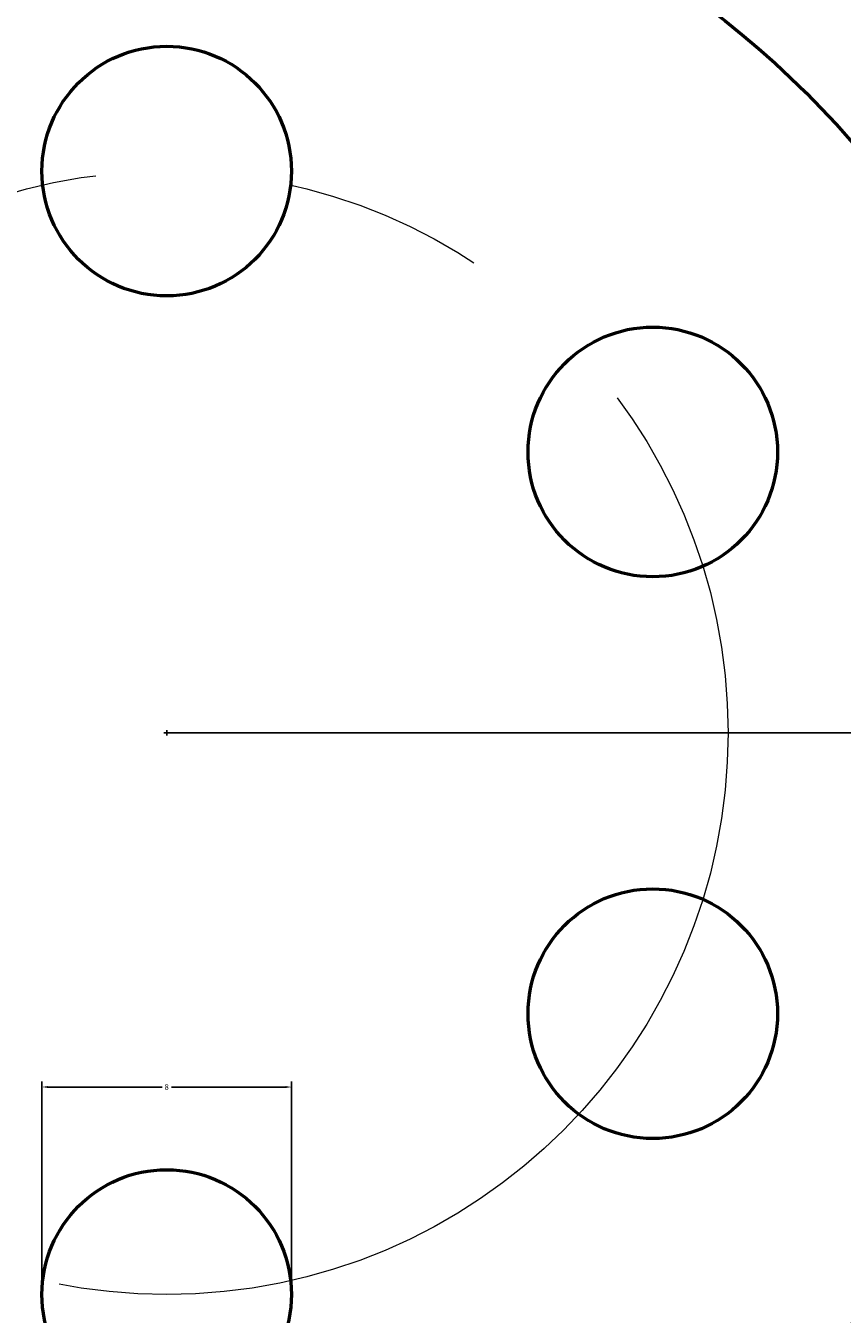
# Model space of a CAD drawing. Units: inches. Extents: x -11 to 126, y -62 to 82.
# Tile 4 of 10: x 55 to 81, y -40 to 1. Entities that reach past the tile are written whole.
import ezdxf

# ---------------------------------------------------------------- set-up
doc = ezdxf.new("R2010")
doc.units = ezdxf.units.IN
doc.header["$MEASUREMENT"] = 0
doc.linetypes.add('CENTER', pattern=[50.8, 31.75, -6.35, 6.35, -6.35])
for name, color, linetype, lineweight in [('M-CNTR', 4, 'CENTER', 18), ('M-DIMS', 2, 'Continuous', 18), ('M-OUTL', 7, 'Continuous', 50)]:
    doc.layers.add(name, color=color, linetype=linetype, lineweight=lineweight)
doc.styles.get("Standard").update_dxf_attribs({"font": 'arial.ttf'})
doc.dimstyles.get("Standard").update_dxf_attribs({"dimtxt": 0.18, "dimasz": 0.18, "dimexe": 0.18, "dimexo": 0.0625, "dimgap": 0.09, "dimtad": 0, "dimtih": 1, "dimtoh": 1, "dimdec": 4, "dimzin": 0, "dimdsep": 46, "dimtxsty": 'Standard', "dimcen": 0.09, "dimadec": 0, "dimazin": 0, "dimtfac": 1, "dimtdec": 4, "dimtofl": 0, "dimtmove": 0, "dimatfit": 3, "dimfxl": 1, "dimtolj": 1, "dimtzin": 0, "dimarcsym": 0})

# ---------------------------------------------------------------- blocks, each defined once
blk = doc.blocks.new('*U3')
blk.add_circle((0, 0), 4)
blk = doc.blocks.new('*U4')
at = {"layer": 'M-OUTL', "color": 0, "linetype": 'ByBlock', "lineweight": -2, "transparency": 16777216}
blk.add_blockref('*U3', (59.232, -3.646), dxfattribs=at)
for p, rotation in [((74.82, -12.646), 300), ((74.82, -30.646), 240), ((59.232, -39.646), 180)]:
    blk.add_blockref('*U3', p, dxfattribs=dict(at, rotation=rotation))
blk = doc.blocks.new('*D5')
at = {"layer": 'Defpoints', "color": 0, "transparency": 16777216}
for p in [(119.232, 12.354), (-0.749, 11.479), (119.232, -57.296)]:
    blk.add_point(p, dxfattribs=at)
at = {"layer": 'M-DIMS', "color": 0, "lineweight": -2, "transparency": 16777216}
for p, q in [((119.232, 12.292), (119.232, -57.476)), ((-0.749, 11.416), (-0.749, -57.476)), ((-0.569, -57.296), (58.786, -57.296)), ((119.052, -57.296), (59.696, -57.296))]:
    blk.add_line(p, q, dxfattribs=at)
at = {"layer": 'M-DIMS', "color": 0, "transparency": 16777216}
for points in [[(-0.569, -57.266), (-0.569, -57.326), (-0.749, -57.296)], [(119.052, -57.266), (119.052, -57.326), (119.232, -57.296)]]:
    blk.add_solid(points, dxfattribs=at)
at = {"layer": 'M-DIMS', "color": 0, "transparency": 16777216, "insert": (59.241, -57.296), "char_height": 0.18, "attachment_point": 5}
blk.add_mtext('\\A1;119.98', dxfattribs=at)
blk = doc.blocks.new('*D6')
at = {"layer": 'Defpoints', "color": 0, "transparency": 16777216}
for p in [(-7.399, 75.354), (59.232, 75.354), (59.232, -50.646)]:
    blk.add_point(p, dxfattribs=at)
at = {"layer": 'M-DIMS', "color": 0, "lineweight": -2, "transparency": 16777216}
for p, q in [((59.169, 75.354), (-7.579, 75.354)), ((-7.399, 75.174), (-7.399, 12.536)), ((-7.399, -50.466), (-7.399, 12.172)), ((59.169, -50.646), (-7.579, -50.646))]:
    blk.add_line(p, q, dxfattribs=at)
at = {"layer": 'M-DIMS', "color": 0, "transparency": 16777216}
for points in [[(-7.429, 75.174), (-7.369, 75.174), (-7.399, 75.354)], [(-7.429, -50.466), (-7.369, -50.466), (-7.399, -50.646)]]:
    blk.add_solid(points, dxfattribs=at)
at = {"layer": 'M-DIMS', "color": 0, "transparency": 16777216, "insert": (-7.399, 12.354), "char_height": 0.18, "attachment_point": 5}
blk.add_mtext('\\A1;126', dxfattribs=at)
blk = doc.blocks.new('*D9')
at = {"layer": 'Defpoints', "color": 0, "transparency": 16777216}
for p in [(99.232, 12.354), (125.882, 12.354), (59.232, -21.646)]:
    blk.add_point(p, dxfattribs=at)
at = {"layer": 'M-DIMS', "color": 0, "lineweight": -2, "transparency": 16777216}
for p, q in [((99.294, 12.354), (126.062, 12.354)), ((125.882, 12.174), (125.882, -4.464)), ((125.882, -21.466), (125.882, -4.828)), ((59.294, -21.646), (126.062, -21.646))]:
    blk.add_line(p, q, dxfattribs=at)
at = {"layer": 'M-DIMS', "color": 0, "transparency": 16777216}
for points in [[(125.852, 12.174), (125.912, 12.174), (125.882, 12.354)], [(125.852, -21.466), (125.912, -21.466), (125.882, -21.646)]]:
    blk.add_solid(points, dxfattribs=at)
at = {"layer": 'M-DIMS', "color": 0, "transparency": 16777216, "insert": (125.882, -4.646), "char_height": 0.18, "attachment_point": 5}
blk.add_mtext('\\A1;34', dxfattribs=at)
blk = doc.blocks.new('*D12')
at = {"layer": 'Defpoints', "color": 0, "transparency": 16777216}
for p in [(63.232, -32.996), (55.232, -39.646), (63.232, -39.646)]:
    blk.add_point(p, dxfattribs=at)
at = {"layer": 'M-DIMS', "color": 0, "lineweight": -2, "transparency": 16777216}
for p, q in [((55.232, -39.583), (55.232, -32.816)), ((55.412, -32.996), (59.082, -32.996)), ((63.052, -32.996), (59.381, -32.996)), ((63.232, -39.583), (63.232, -32.816))]:
    blk.add_line(p, q, dxfattribs=at)
at = {"layer": 'M-DIMS', "color": 0, "transparency": 16777216}
for points in [[(55.412, -32.966), (55.412, -33.026), (55.232, -32.996)], [(63.052, -32.966), (63.052, -33.026), (63.232, -32.996)]]:
    blk.add_solid(points, dxfattribs=at)
at = {"layer": 'M-DIMS', "color": 0, "transparency": 16777216, "insert": (59.232, -32.996), "char_height": 0.18, "attachment_point": 5}
blk.add_mtext('\\A1;8', dxfattribs=at)
blk = doc.blocks.new('*D13')
at = {"layer": 'Defpoints', "color": 0, "transparency": 16777216}
for p in [(73.731, 3.469), (44.732, -46.761)]:
    blk.add_point(p, dxfattribs=at)
at = {"layer": 'M-DIMS', "color": 0, "lineweight": -2, "transparency": 16777216}
for p, q in [((59.142, -21.646), (59.322, -21.646)), ((59.232, -21.736), (59.232, -21.556)), ((36.032, -61.83), (44.642, -46.917)), ((35.852, -61.83), (36.032, -61.83))]:
    blk.add_line(p, q, dxfattribs=at)
at = {"layer": 'M-DIMS', "color": 0, "transparency": 16777216}
blk.add_solid([(44.616, -46.902), (44.668, -46.932), (44.732, -46.761)], dxfattribs=at)
at = {"layer": 'M-DIMS', "color": 0, "transparency": 16777216, "insert": (35.345, -61.83), "char_height": 0.18, "attachment_point": 5}
blk.add_mtext('\\A1;2X ∅58', dxfattribs=at)
blk = doc.blocks.new('*D15')
at = {"layer": 'Defpoints', "color": 0, "transparency": 16777216}
for p in [(41.232, -21.646), (77.232, -21.645)]:
    blk.add_point(p, dxfattribs=at)
at = {"layer": 'M-DIMS', "color": 0, "lineweight": -2, "transparency": 16777216}
for p, q in [((30.432, -21.646), (41.052, -21.646)), ((59.142, -21.646), (59.322, -21.646)), ((59.232, -21.736), (59.232, -21.556))]:
    blk.add_line(p, q, dxfattribs=at)
at = {"layer": 'M-DIMS', "color": 0, "transparency": 16777216}
blk.add_solid([(41.052, -21.616), (41.052, -21.676), (41.232, -21.646)], dxfattribs=at)
at = {"layer": 'M-DIMS', "color": 0, "transparency": 16777216, "insert": (30.115, -21.646), "char_height": 0.18, "attachment_point": 5}
blk.add_mtext('\\A1;∅36', dxfattribs=at)

msp = doc.modelspace()

# ---------------------------------------------------------------- linework, layer by layer
at = {"layer": 'M-CNTR'}
msp.add_circle((59.232, -21.646), 18, dxfattribs=at)
at = {"layer": 'M-OUTL'}
msp.add_circle((59.232, -21.646), 29, dxfattribs=at)

# ---------------------------------------------------------------- block references
msp.add_blockref('*U4', (0, 0), dxfattribs=at)

# ---------------------------------------------------------------- dimensions: what is measured, and where the dimension line sits
at = {"layer": 'M-DIMS'}
for base, p1, p2, picture, middle in [((-7.399, 75.354), (59.232, -50.646), (59.232, 75.354), '*D6', (-7.399, 12.354)), ((125.882, 12.354), (59.232, -21.646), (99.232, 12.354), '*D9', (125.882, -4.646))]:
    dim = msp.add_linear_dim(base=base, p1=p1, p2=p2, angle=90, dimstyle='Standard', override={"dimdec": 0, "dimlfac": 1, "dimrnd": 0, "dimzin": 0, "dimdsep": 46, "dimlunit": 2}, dxfattribs=at)
    dim.commit()
    dim.dimension.update_dxf_attribs({"geometry": picture, "text_midpoint": middle})
for base, p1, p2, override, picture, middle in [((119.232, -57.296), (-0.749, 11.479), (119.232, 12.354), {"dimdec": 2, "dimlfac": 1, "dimrnd": 0, "dimzin": 0, "dimdsep": 46, "dimlunit": 2}, '*D5', (59.241, -57.296)), ((63.232, -32.996), (55.232, -39.646), (63.232, -39.646), {"dimdec": 0, "dimlfac": 1, "dimrnd": 0, "dimzin": 0, "dimdsep": 46, "dimlunit": 2}, '*D12', (59.232, -32.996))]:
    dim = msp.add_linear_dim(base=base, p1=p1, p2=p2, dimstyle='Standard', override=override, dxfattribs=at)
    dim.commit()
    dim.dimension.update_dxf_attribs({"geometry": picture, "text_midpoint": middle})
dim = msp.add_diameter_dim_2p(p1=(73.731, 3.469), p2=(44.732, -46.761), text='2X <>', dimstyle='Standard', override={"dimdec": 0, "dimlfac": 1, "dimrnd": 0, "dimzin": 0, "dimdsep": 46, "dimlunit": 2}, dxfattribs=at)
dim.commit()
dim.dimension.update_dxf_attribs({"geometry": '*D13', "text_midpoint": (35.345, -61.83), "dimtype": 163})
dim = msp.add_diameter_dim_2p(p1=(77.232, -21.645), p2=(41.232, -21.646), dimstyle='Standard', override={"dimdec": 0, "dimlfac": 1, "dimrnd": 0, "dimzin": 0, "dimdsep": 46, "dimlunit": 2}, dxfattribs=at)
dim.commit()
dim.dimension.update_dxf_attribs({"geometry": '*D15', "text_midpoint": (30.432, -21.646), "dimtype": 163})

doc.saveas('drawing.dxf')
